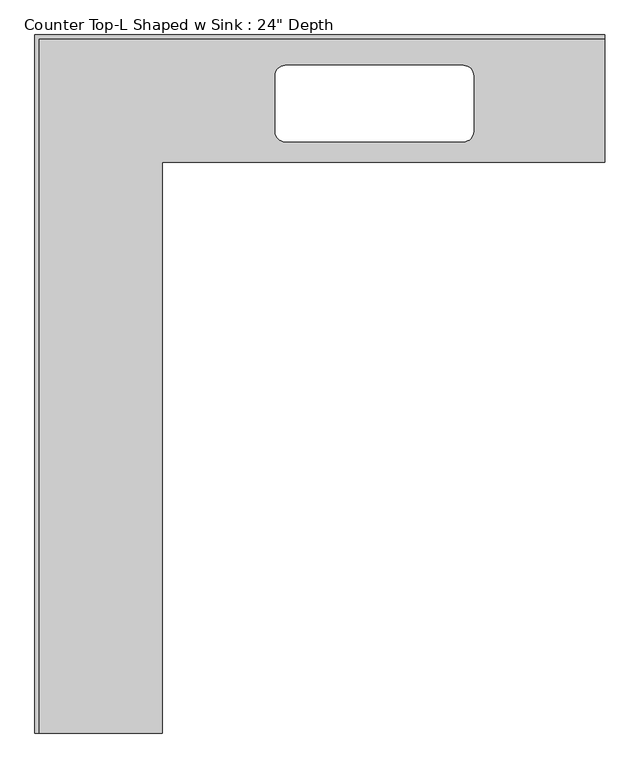
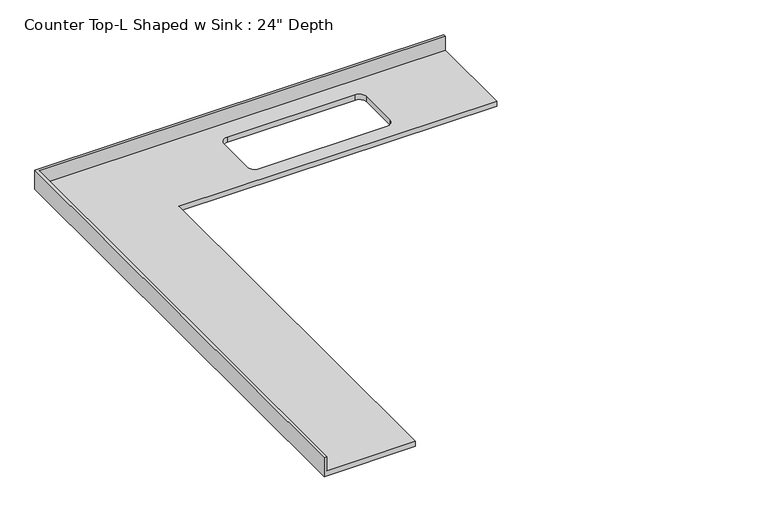
"""IFC4 building model written with IfcOpenShell, lengths in millimetres: furniture geometry."""

from ifc_helpers import new_model, si_unit, frame, origin, place, context, project, spatial, polyline, circle_curve, source, transform, mapped, element, save
from ifc_brep_helpers import plane_surface, revolved_surface, advanced_brep


def furniture_bc267eac(model_context):
    return source(origin(), model_context, "Body", "AdvancedBrep", [
        advanced_brep(
        [(-565.4622951, -3485.5965233, 914.4), (-565.4622951, -635.0, 914.4), (1644.3377049, -635.0, 914.4), (1644.3377049, -19.05, 914.4), (-1181.4122951, -19.05, 914.4), (-1181.4122951, -3485.5965233, 914.4), (938.4904422, -152.4, 914.4), (989.2904422, -203.2, 914.4), (989.2904422, -482.6, 914.4), (938.4904422, -533.4, 914.4), (49.4904422, -533.4, 914.4), (-1.3095578, -482.6, 914.4), (-1.3095578, -203.2, 914.4), (49.4904422, -152.4, 914.4), (1644.3377049, 0.0, 876.3), (1644.3377049, -635.0, 876.3), (-565.4622951, -635.0, 876.3), (-565.4622951, -3485.5965233, 876.3), (-1200.4622951, -3485.5965233, 876.3), (-1200.4622951, 0.0, 876.3), (938.4904422, -152.4, 876.3), (49.4904422, -152.4, 876.3), (-1.3095578, -203.2, 876.3), (-1.3095578, -482.6, 876.3), (49.4904422, -533.4, 876.3), (938.4904422, -533.4, 876.3), (989.2904422, -482.6, 876.3), (989.2904422, -203.2, 876.3), (-1200.4622951, 0.0, 1016.0), (1644.3377049, 0.0, 1016.0), (-1200.4622951, -3485.5965233, 1016.0), (-1181.4122951, -3485.5965233, 1016.0), (1644.3377049, -19.05, 1016.0), (-1181.4122951, -19.05, 1016.0)],
        [
            (0, 1),
            (1, 2),
            (2, 3),
            (3, 4),
            (4, 5),
            (5, 0),
            (6, 7, circle_curve(frame((938.4904422, -203.2, 914.4), z_axis=(0.0, 0.0, -1.0), x_axis=(1.0, 0.0, 0.0)), 50.8)),
            (7, 8),
            (8, 9, circle_curve(frame((938.4904422, -482.6, 914.4), z_axis=(0.0, 0.0, -1.0), x_axis=(1.0, 0.0, 0.0)), 50.8)),
            (9, 10),
            (10, 11, circle_curve(frame((49.4904422, -482.6, 914.4), z_axis=(0.0, 0.0, -1.0), x_axis=(1.0, 0.0, 0.0)), 50.8)),
            (11, 12),
            (12, 13, circle_curve(frame((49.4904422, -203.2, 914.4), z_axis=(0.0, 0.0, -1.0), x_axis=(1.0, 0.0, 0.0)), 50.8)),
            (13, 6),
            (14, 15),
            (15, 16),
            (16, 17),
            (17, 18),
            (18, 19),
            (19, 14),
            (20, 21),
            (21, 22, circle_curve(frame((49.4904422, -203.2, 876.3), z_axis=(0.0, 0.0, 1.0), x_axis=(1.0, 0.0, 0.0)), 50.8)),
            (22, 23),
            (23, 24, circle_curve(frame((49.4904422, -482.6, 876.3), z_axis=(0.0, 0.0, 1.0), x_axis=(1.0, 0.0, 0.0)), 50.8)),
            (24, 25),
            (25, 26, circle_curve(frame((938.4904422, -482.6, 876.3), z_axis=(0.0, 0.0, 1.0), x_axis=(1.0, 0.0, 0.0)), 50.8)),
            (26, 27),
            (27, 20, circle_curve(frame((938.4904422, -203.2, 876.3), z_axis=(0.0, 0.0, 1.0), x_axis=(1.0, 0.0, 0.0)), 50.8)),
            (19, 28),
            (28, 29),
            (29, 14),
            (18, 30),
            (30, 28),
            (17, 0),
            (5, 31),
            (31, 30),
            (16, 1),
            (15, 2),
            (29, 32),
            (32, 3),
            (6, 20),
            (27, 7),
            (26, 8),
            (25, 9),
            (24, 10),
            (23, 11),
            (22, 12),
            (21, 13),
            (31, 33),
            (33, 32),
            (33, 4),
        ],
        [
            plane_surface(frame((-1200.4622951, 0.0, 914.4), z_axis=(0.0, 0.0, 1.0), x_axis=(-1.0, 0.0, 0.0))),
            plane_surface(frame((-1200.4622951, 0.0, 876.3), z_axis=(0.0, 0.0, -1.0), x_axis=(1.0, 0.0, 0.0))),
            plane_surface(frame((1644.3377049, 0.0, 914.4), z_axis=(0.0, 1.0, 0.0), x_axis=(0.0, 0.0, -1.0))),
            plane_surface(frame((-1200.4622951, 0.0, 914.4), z_axis=(-1.0, 0.0, 0.0), x_axis=(0.0, 0.0, -1.0))),
            plane_surface(frame((-1200.4622951, -3485.5965233, 914.4), z_axis=(0.0, -1.0, 0.0), x_axis=(0.0, 0.0, -1.0))),
            plane_surface(frame((-565.4622951, -3485.5965233, 914.4), z_axis=(1.0, 0.0, 0.0), x_axis=(0.0, 0.0, -1.0))),
            plane_surface(frame((-565.4622951, -635.0, 914.4), z_axis=(0.0, -1.0, 0.0), x_axis=(0.0, 0.0, -1.0))),
            plane_surface(frame((1644.3377049, -635.0, 914.4), z_axis=(1.0, 0.0, 0.0), x_axis=(0.0, 0.0, -1.0))),
            revolved_surface(polyline([(989.2904421999999, -203.2, 876.3), (989.2904421999999, -203.2, 914.4)]), (938.4904422, -203.2, 0.0), (0.0, 0.0, -1.0)),
            plane_surface(frame((989.2904422, -203.2, 914.4), z_axis=(-1.0, 0.0, 0.0), x_axis=(0.0, 0.0, -1.0))),
            revolved_surface(polyline([(989.2904421999999, -482.6, 876.3), (989.2904421999999, -482.6, 914.4)]), (938.4904422, -482.6, 0.0), (0.0, 0.0, -1.0)),
            plane_surface(frame((938.4904422, -533.4, 914.4), z_axis=(0.0, 1.0, 0.0), x_axis=(0.0, 0.0, -1.0))),
            revolved_surface(polyline([(100.2904422, -482.6, 876.3), (100.2904422, -482.6, 914.4)]), (49.4904422, -482.6, 0.0), (0.0, 0.0, -1.0)),
            plane_surface(frame((-1.3095578, -482.6, 914.4), z_axis=(1.0, 0.0, 0.0), x_axis=(0.0, 0.0, -1.0))),
            revolved_surface(polyline([(100.2904422, -203.2, 876.3), (100.2904422, -203.2, 914.4)]), (49.4904422, -203.2, 0.0), (0.0, 0.0, -1.0)),
            plane_surface(frame((49.4904422, -152.4, 914.4), z_axis=(0.0, -1.0, 0.0), x_axis=(0.0, 0.0, -1.0))),
            plane_surface(frame((-1200.4622951, 0.0, 1016.0), z_axis=(0.0, 0.0, 1.0), x_axis=(0.0, -1.0, 0.0))),
            plane_surface(frame((-1200.4622951, -19.05, 1016.0), z_axis=(0.0, -1.0, 0.0), x_axis=(0.0, 0.0, -1.0))),
            plane_surface(frame((-1181.4122951, -3485.5965233, 1016.0), z_axis=(1.0, 0.0, 0.0), x_axis=(0.0, 0.0, -1.0))),
        ],
        [
            (0, [[1, 2, 3, 4, 5, 6], [7, 8, 9, 10, 11, 12, 13, 14]]),
            (1, [[15, 16, 17, 18, 19, 20], [21, 22, 23, 24, 25, 26, 27, 28]]),
            (2, [[-20, 29, 30, 31]]),
            (3, [[-19, 32, 33, -29]]),
            (4, [[-32, -18, 34, -6, 35, 36]]),
            (5, [[-1, -34, -17, 37]]),
            (6, [[-2, -37, -16, 38]]),
            (7, [[-15, -31, 39, 40, -3, -38]]),
            (8, [[-7, 41, -28, 42]]),
            (9, [[-8, -42, -27, 43]]),
            (10, [[-9, -43, -26, 44]]),
            (11, [[-10, -44, -25, 45]]),
            (12, [[-11, -45, -24, 46]]),
            (13, [[-12, -46, -23, 47]]),
            (14, [[-13, -47, -22, 48]]),
            (15, [[-14, -48, -21, -41]]),
            (16, [[-33, -36, 49, 50, -39, -30]]),
            (17, [[-40, -50, 51, -4]]),
            (18, [[-49, -35, -5, -51]]),
        ],
    ),
    ])


if __name__ == "__main__":
    model = new_model("IFC4")
    model_context = context("Model", 3, world=origin())
    ifc_project = project(units=[si_unit("LENGTHUNIT", "METRE", prefix="MILLI")], contexts=[model_context])
    site = spatial("IfcSite", under=ifc_project)
    building = spatial("IfcBuilding", under=site)
    placement = place(None, origin())
    furniture_shape = furniture_bc267eac(model_context)
    element("IfcFurniture", 1, ObjectType="Counter Top-L Shaped w Sink : 24\" Depth", at=placement, inside=building, context=model_context, shape_type="MappedRepresentation", body=[
        mapped(furniture_shape, transform((0.0, 0.0, 0.0), x_axis=(1.0, 0.0, 0.0), y_axis=(0.0, 1.0, 0.0), z_axis=(0.0, 0.0, 1.0))),
    ])
    save(model, "model.ifc")

# Revit data of these elements
# Type "Counter Top-L Shaped w Sink : 24\" Depth"
#   Assembly Code = "C1030400"
#   Counter Thickness = 0' - 1 1/2"
#   Depth = 2' - 1"
#   Height = 3' - 0"
#   Length - Leg 1 [instance default] = 8' - 0"
#   Length - Leg 2 [instance default] = 6' - 0"
#   Sink Location [instance default] = 3' - 0"
#   Sink Location To Wall [instance default] = 0' - 6"
#   Sink Opening Depth [instance default] = 1' - 3"
#   Sink Opening Width [instance default] = 3' - 3"
#   Counter Top Material = none
#   Default Elevation = 0
# Element 1 (IfcFurniture, "Counter Top-L Shaped w Sink : 24\" Depth")
#   Length - Leg 1 = 9' - 4"
#   Length - Leg 2 = 11' - 5.22821"
#   Sink Location = 3' - 11.21074"
#   Materials on its faces: "Counter Top"
# Materials
#   "Counter Top": class "Wood", colour RGB 226 177 128, transparency 0
